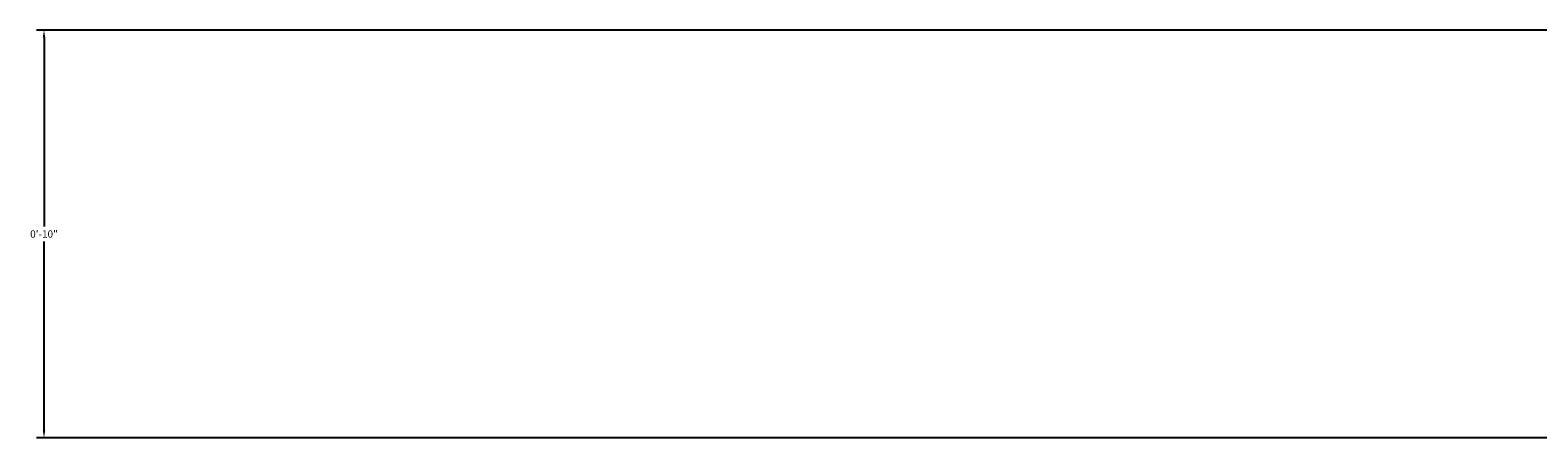
# Model space of a CAD drawing. Units: inches. Extents: x -5 to 482, y -460 to 66.
# Tile 2 of 31: x -5 to 32, y -386 to -376. Entities that reach past the tile are written whole.
import ezdxf

# ---------------------------------------------------------------- set-up
doc = ezdxf.new("R2010")
doc.units = ezdxf.units.IN
doc.header["$MEASUREMENT"] = 0
doc.layers.add('A-ANNO-DIMS', color=2, linetype='Continuous', lineweight=18)
doc.styles.get("Standard").update_dxf_attribs({"font": 'arial.ttf'})
doc.dimstyles.get("Standard").update_dxf_attribs({"dimtxt": 0.18, "dimasz": 0.18, "dimexe": 0.18, "dimexo": 0.0625, "dimgap": 0.09, "dimtad": 0, "dimtih": 1, "dimtoh": 1, "dimdec": 0, "dimzin": 0, "dimdsep": 46, "dimlunit": 3, "dimtxsty": 'Standard', "dimcen": 0.09, "dimadec": 0, "dimazin": 0, "dimtfac": 1, "dimtdec": 0, "dimtofl": 0, "dimtmove": 0, "dimatfit": 3, "dimfxl": 1, "dimtolj": 1, "dimtzin": 0, "dimarcsym": 0})

# ---------------------------------------------------------------- blocks, each defined once
blk = doc.blocks.new('*D72')
at = {"layer": 'A-ANNO-DIMS', "color": 0, "lineweight": -2, "transparency": 16777216}
for p, q in [((144.314, -375.861), (-4.903, -375.861)), ((-4.723, -376.041), (-4.723, -380.679)), ((-4.723, -385.681), (-4.723, -381.043)), ((144.314, -385.861), (-4.903, -385.861))]:
    blk.add_line(p, q, dxfattribs=at)
at = {"layer": 'A-ANNO-DIMS', "color": 0, "transparency": 16777216}
for points in [[(-4.753, -376.041), (-4.693, -376.041), (-4.723, -375.861)], [(-4.753, -385.681), (-4.693, -385.681), (-4.723, -385.861)]]:
    blk.add_solid(points, dxfattribs=at)
at = {"layer": 'Defpoints', "color": 0, "transparency": 16777216}
for p in [(144.377, -375.861), (-4.723, -385.861), (144.377, -385.861)]:
    blk.add_point(p, dxfattribs=at)
at = {"layer": 'A-ANNO-DIMS', "color": 0, "transparency": 16777216, "insert": (-4.723, -380.861), "char_height": 0.18, "attachment_point": 5}
blk.add_mtext('\\A1;0\'-10"', dxfattribs=at)

msp = doc.modelspace()

# ---------------------------------------------------------------- dimensions: what is measured, and where the dimension line sits
at = {"layer": 'A-ANNO-DIMS'}
dim = msp.add_linear_dim(base=(-4.723, -385.861), p1=(144.377, -375.861), p2=(144.377, -385.861), angle=90, dimstyle='Standard', override={"dimdec": 1, "dimlfac": 1, "dimrnd": 0, "dimzin": 1, "dimdsep": 46, "dimlunit": 4, "dimfrac": 2}, dxfattribs=at)
dim.commit()
dim.dimension.update_dxf_attribs({"geometry": '*D72', "text_midpoint": (-4.723, -380.861)})

doc.saveas('drawing.dxf')
